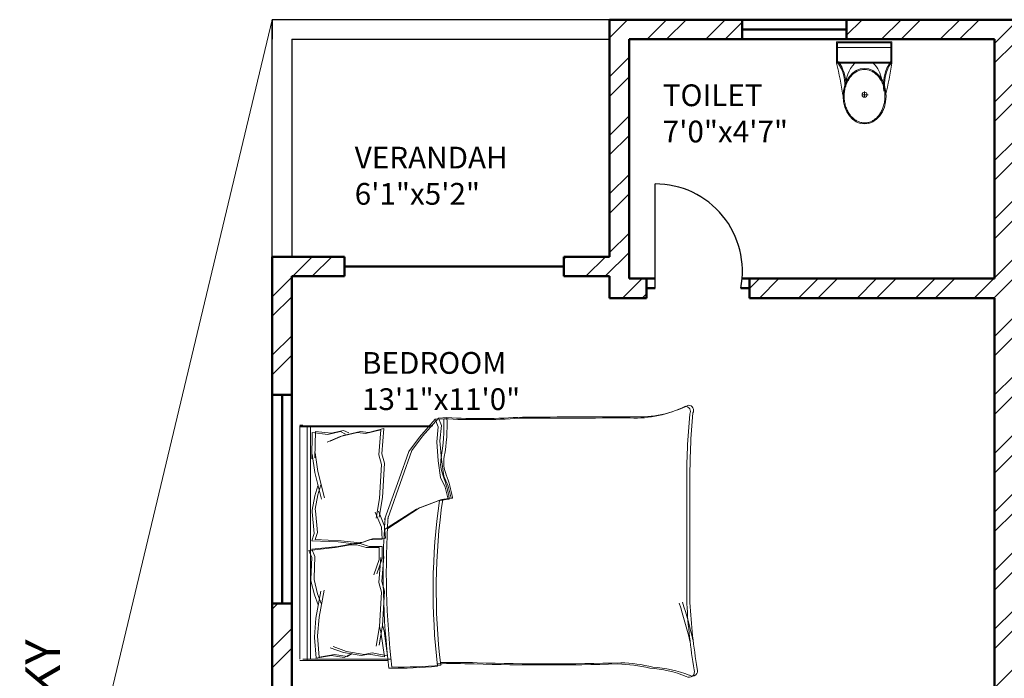
# Model space of a CAD drawing. Units: inches. Extents: x 1901 to 2863, y 888 to 2433.
# Tile 78 of 91: x 2381 to 2608, y 2123 to 2274. Entities that reach past the tile are written whole.
import ezdxf

# ---------------------------------------------------------------- set-up
doc = ezdxf.new("R2010")
doc.units = ezdxf.units.IN
for name, color, linetype, lineweight in [('A-ANNO-SYMB', 8, 'Continuous', 13), ('A-AREA-IDEN', 7, 'Continuous', 18), ('A-DOOR', 4, 'Continuous', 25), ('A-FLOR-FIXT', 9, 'Continuous', 18), ('A-FLOR-HRAL', 41, 'Continuous', 25), ('A-FURN', 8, 'Continuous', 18), ('A-WALL', 7, 'Continuous', 50), ('A-WALL-PATT', 8, 'Continuous', 13)]:
    doc.layers.add(name, color=color, linetype=linetype, lineweight=lineweight)
doc.styles.get("Standard").update_dxf_attribs({"font": 'arial.ttf'})

# ---------------------------------------------------------------- blocks, each defined once
blk = doc.blocks.new('A$C31115884')
for p, q in [((283.1, 497.7), (223.4, 497.7)), ((257.5, 466.4), (257.5, 523.2)), ((0, 200), (0, 0)), ((520, 200), (0, 200)), ((10, 190), (10, 10)), ((510, 190), (10, 190)), ((510, 10), (510, 190)), ((520, 0), (520, 200)), ((510, 54.5), (0, 54.5)), ((10, 10), (510, 10)), ((0, 0), (520, 0))]:
    blk.add_line(p, q)
blk.add_circle((255.6, 496.4), 23.6)
for centre, radius, start, end in [((2777.7, -204.6), 2807, 165.4549, 171.71327), ((-294.5, 403.3), 364.7, 324.20913, 9.34987), ((-294.5, 403.3), 374.7, 324.20913, 9.34987), ((805.8, 403.3), 364.7, 170.65013, 215.79087), ((3237, 905), 2807, 188.28673, 194.5451), ((139.5, 406.2), 293.5, 315.84364, 2.65635), ((805.8, 403.3), 374.7, 179.20365, 215.79087), ((383.6, 406.2), 293.5, 190.27735, 224.15636)]:
    blk.add_arc(centre, radius, start, end)
blk.add_ellipse((256.2, 509.9), major_axis=(0, -260.7), ratio=0.772727)
blk.add_open_spline([(256.2, 259.2), (263.1, 259.2), (270, 259.7), (287.8, 262.3), (298.7, 265.1), (319.9, 273.1), (330.2, 278.4), (350.1, 291.1), (359.7, 298.7), (377.7, 315.9), (386.2, 325.5), (401.7, 346.6), (408.8, 358.1), (421.3, 382.5), (426.8, 395.5), (435.9, 422.4), (439.5, 436.4), (444.8, 465.1), (446.5, 479.7), (447.9, 509.2), (447.6, 524), (445, 553.3), (442.7, 567.8), (436.3, 596), (432.1, 609.7), (421.9, 636), (416, 648.6), (402.5, 672.1), (395, 683), (378.6, 703), (369.8, 712.1), (351.1, 728), (341.3, 734.8), (320.9, 746.2), (310.4, 750.7), (288.9, 757.3), (278, 759.4), (256, 761), (245, 760.6), (223.1, 757.2), (212.3, 754.3), (191.1, 746.1), (180.8, 740.7), (160.9, 727.8), (151.4, 720.1), (133.5, 702.7), (125.1, 693), (109.6, 671.7), (102.6, 660.2), (90.2, 635.7), (84.9, 622.7), (76, 595.6), (72.4, 581.6), (67.2, 552.9), (65.6, 538.2), (64.4, 508.8), (64.8, 494), (67.5, 464.7), (69.9, 450.2), (76.6, 422), (80.8, 408.3), (91.1, 382.2), (97.2, 369.7), (110.8, 346.3), (118.4, 335.4), (134.8, 315.6), (143.7, 306.7), (162.4, 290.9), (172.3, 284.2), (192.8, 273), (203.3, 268.6), (224.8, 262.2), (235.8, 260.2), (249.9, 259.3), (253, 259.2), (256.2, 259.2)], degree=3, knots=[0, 0, 0, 0, 0.110105, 0.110105, 0.285049, 0.285049, 0.459994, 0.459994, 0.634938, 0.634938, 0.809882, 0.809882, 0.984827, 0.984827, 1.159771, 1.159771, 1.334715, 1.334715, 1.50966, 1.50966, 1.684604, 1.684604, 1.859549, 1.859549, 2.034493, 2.034493, 2.209437, 2.209437, 2.384382, 2.384382, 2.559326, 2.559326, 2.73427, 2.73427, 2.909215, 2.909215, 3.084159, 3.084159, 3.259103, 3.259103, 3.434048, 3.434048, 3.608992, 3.608992, 3.783936, 3.783936, 3.958881, 3.958881, 4.133825, 4.133825, 4.30877, 4.30877, 4.483714, 4.483714, 4.658658, 4.658658, 4.833603, 4.833603, 5.008547, 5.008547, 5.183491, 5.183491, 5.358436, 5.358436, 5.53338, 5.53338, 5.708324, 5.708324, 5.883269, 5.883269, 6.058213, 6.058213, 6.233158, 6.233158, 6.283185, 6.283185, 6.283185, 6.283185])
blk = doc.blocks.new('BED-DOUBLE')
for p, q in [((31.18, 59.32), (27.53, 55.16)), ((31.18, 59.32), (27.53, 55.16)), ((31.9, 59.58), (28.25, 55.42)), ((31.9, 59.58), (28.25, 55.42)), ((33.14, 59.41), (31.18, 59.32, 4.35)), ((33.14, 59.41), (31.18, 59.32, 4.35)), ((31.87, 57.59), (31.18, 59.32)), ((31.87, 57.59), (31.18, 59.32)), ((33.85, 59.67), (31.9, 59.58, 4.35)), ((33.85, 59.67), (31.9, 59.58, 4.35)), ((32.59, 57.85), (31.9, 59.58)), ((32.59, 57.85), (31.9, 59.58)), ((0.03, 57.78), (0.03, 4.12)), ((0.74, 57.78), (30.62, 57.78)), ((0.74, 57.78), (30.62, 57.78)), ((7.22, 56.06), (10.11, 56.73)), ((7.22, 56.06), (10.11, 56.73)), ((10.11, 56.73), (11.28, 56.15)), ((10.11, 56.73), (11.28, 56.15)), ((18.63, 56.89), (15.11, 56.01)), ((18.63, 56.88), (15.11, 56.01)), ((19.35, 57.14), (15.83, 56.27)), ((19.35, 57.14), (15.83, 56.27)), ((18.18, 51.12), (18.63, 56.89)), ((18.18, 51.12), (18.63, 56.88)), ((18.9, 51.38), (19.35, 57.14)), ((18.9, 51.38), (19.35, 57.14)), ((31.53, 54.12), (31.87, 57.59)), ((31.53, 54.12), (31.87, 57.59)), ((32.24, 54.37), (32.59, 57.85)), ((32.24, 54.37), (32.59, 57.85)), ((2.9, 56.23), (2.79, 50.16)), ((2.9, 56.23), (2.79, 50.16)), ((2.9, 56.23), (6.5, 55.8)), ((2.9, 56.23), (6.5, 55.8)), ((3.61, 56.48), (3.51, 50.42)), ((3.61, 56.48), (3.51, 50.42)), ((3.61, 56.48), (7.22, 56.06)), ((3.61, 56.48), (7.22, 56.06)), ((9.3, 55.33), (6.29, 54)), ((9.3, 55.33), (6.29, 54)), ((6.5, 55.8), (9.39, 56.47)), ((6.5, 55.8), (9.39, 56.47)), ((10.01, 55.58), (7.01, 54.26)), ((10.01, 55.58), (7.01, 54.26)), ((13.31, 56.23), (9.3, 55.33)), ((13.31, 56.23), (9.3, 55.33)), ((9.39, 56.47), (10.56, 55.89)), ((9.39, 56.47), (10.56, 55.89)), ((14.02, 56.48), (10.01, 55.58)), ((14.02, 56.48), (10.01, 55.58)), ((15.11, 56.01), (13.31, 56.23)), ((15.11, 56.01), (13.31, 56.23)), ((15.83, 56.27), (14.02, 56.48)), ((15.83, 56.27), (14.02, 56.48)), ((27.53, 55.16), (25.1, 51.86)), ((27.53, 55.16), (25.1, 51.86)), ((28.25, 55.42), (25.81, 52.11)), ((28.25, 55.42), (25.81, 52.11)), ((32.59, 50.03), (32.24, 54.37)), ((32.59, 50.03), (32.24, 54.37)), ((25.81, 52.11), (23.55, 45.85)), ((25.81, 52.11), (23.55, 45.85)), ((31.87, 49.77), (31.53, 54.12)), ((31.87, 49.77), (31.53, 54.12)), ((2.79, 50.16), (2.88, 51.29)), ((2.79, 50.16), (2.88, 51.29)), ((2.88, 51.29), (3.47, 47.02)), ((2.88, 51.29), (3.47, 47.02)), ((3.51, 50.42), (3.6, 51.54)), ((3.51, 50.42), (3.6, 51.54)), ((3.6, 51.54), (4.19, 47.28)), ((3.6, 51.54), (4.19, 47.28)), ((18.81, 48.92), (18.18, 51.12)), ((18.81, 48.92), (18.18, 51.12)), ((19.52, 49.18), (18.9, 51.38)), ((19.52, 49.18), (18.9, 51.38)), ((25.1, 51.86), (22.84, 45.6)), ((25.1, 51.86), (22.84, 45.6)), ((33.11, 46.2), (32.59, 50.03)), ((33.11, 46.2), (32.59, 50.03)), ((18.32, 41.05), (18.81, 48.92)), ((18.32, 41.05), (18.81, 48.92)), ((19.04, 41.31), (19.52, 49.18)), ((19.04, 41.31), (19.52, 49.18)), ((32.39, 45.94), (31.87, 49.77)), ((32.39, 45.94), (31.87, 49.77)), ((3.47, 47.02), (4.99, 40.94)), ((3.47, 47.02), (4.99, 40.94)), ((4.19, 47.28), (5.71, 41.19)), ((4.19, 47.28), (5.71, 41.19)), ((22.84, 45.6), (19.54, 36.24)), ((22.84, 45.6), (19.54, 36.24)), ((23.55, 45.85), (20.26, 36.49)), ((23.55, 45.85), (20.26, 36.49)), ((33.44, 43.68), (32.39, 45.94)), ((33.44, 43.68), (32.39, 45.94)), ((34.15, 43.94), (33.11, 46.2)), ((34.15, 43.94), (33.11, 46.2)), ((4.15, 43.98), (3.48, 41.66)), ((4.15, 43.98), (3.48, 41.66)), ((4.87, 44.23), (4.2, 41.91)), ((4.87, 44.23), (4.2, 41.91)), ((34.13, 40.9), (33.44, 43.68)), ((34.13, 40.9), (33.44, 43.68)), ((34.85, 41.16), (34.15, 43.94)), ((34.85, 41.16), (34.15, 43.94)), ((89, 16.88), (89, 44.51)), ((89, 16.88), (89, 44.51)), ((89.72, 17.13), (89.72, 44.77)), ((89.72, 17.13), (89.72, 44.77)), ((3.48, 41.66), (2.87, 38.37)), ((3.48, 41.66), (2.87, 38.37)), ((4.2, 41.91), (3.59, 38.62)), ((4.2, 41.91), (3.59, 38.62)), ((17.57, 36.53), (18.32, 41.05)), ((17.57, 36.52), (18.32, 41.05)), ((18.29, 36.78), (19.04, 41.31)), ((18.29, 36.78), (19.04, 41.31)), ((27.55, 38.9), (32.59, 40.81)), ((27.55, 38.9), (32.59, 40.81)), ((31.87, 40.55), (34.13, 40.9)), ((31.87, 40.55), (34.13, 40.9)), ((32.59, 40.81), (34.85, 41.16)), ((32.59, 40.81), (34.85, 41.16)), ((3.59, 38.62), (3.62, 38.26)), ((3.59, 38.62), (3.62, 38.26)), ((19.54, 33.94), (26.83, 38.64)), ((19.54, 33.94), (26.83, 38.64)), ((20.26, 34.19), (27.55, 38.9)), ((20.26, 34.19), (27.55, 38.9)), ((26.83, 38.64), (31.87, 40.55)), ((26.83, 38.64), (31.87, 40.55)), ((2.87, 38.37), (2.9, 38.01)), ((2.87, 38.37), (2.9, 38.01)), ((2.9, 38.01), (3.37, 33.03)), ((2.9, 38.01), (3.37, 33.04)), ((3.62, 38.26), (4.09, 33.29)), ((3.62, 38.26), (4.09, 33.29)), ((18.82, 34.49), (17.38, 37.94)), ((18.82, 34.49), (17.38, 37.94)), ((19.54, 34.74), (18.1, 38.19)), ((19.54, 34.74), (18.1, 38.19)), ((18.99, 31.73), (18.82, 34.49)), ((18.99, 31.73), (18.82, 34.49)), ((19.71, 31.99), (19.54, 34.74)), ((19.71, 31.99), (19.54, 34.74)), ((3.37, 33.04), (2.82, 31.37)), ((3.37, 33.03), (2.82, 31.37)), ((4.09, 33.29), (3.54, 31.63)), ((4.09, 33.29), (3.54, 31.63)), ((14.64, 31.02), (16.71, 31.8)), ((14.64, 31.02), (16.71, 31.8)), ((15.99, 31.55), (18.99, 31.73)), ((15.99, 31.55), (18.99, 31.73)), ((16.71, 31.8), (19.71, 31.99)), ((16.71, 31.8), (19.71, 31.99)), ((2.13, 29.14), (8.13, 29.78)), ((2.13, 29.14), (8.13, 29.78)), ((2.82, 31.37), (8.86, 31.1)), ((2.82, 31.37), (8.86, 31.1)), ((2.84, 29.39), (8.85, 30.04)), ((2.84, 29.39), (8.85, 30.04)), ((3.54, 31.63), (9.58, 31.36)), ((3.54, 31.63), (9.58, 31.36)), ((8.13, 29.78), (11.7, 30.43)), ((8.13, 29.78), (11.7, 30.43)), ((8.85, 30.04), (12.42, 30.69)), ((8.85, 30.04), (12.42, 30.69)), ((8.86, 31.1), (12.46, 30.68)), ((8.86, 31.1), (12.46, 30.68)), ((9.58, 31.36), (13.18, 30.93)), ((9.58, 31.36), (13.18, 30.93)), ((11.7, 30.43), (13.16, 30.43)), ((11.7, 30.43), (13.16, 30.43)), ((12.42, 30.69), (13.88, 30.69)), ((12.42, 30.69), (13.88, 30.69)), ((12.46, 30.68), (13.92, 30.77)), ((12.46, 30.68), (13.92, 30.77)), ((13.16, 30.43), (15.28, 29.78)), ((13.16, 30.43), (15.28, 29.78)), ((13.18, 30.93), (14.64, 31.02)), ((13.18, 30.93), (14.64, 31.02)), ((13.88, 30.69), (15.99, 30.04)), ((13.88, 30.69), (15.99, 30.04)), ((13.92, 30.77), (15.99, 31.55)), ((13.92, 30.77), (15.99, 31.55)), ((15.28, 29.78), (18.29, 29.78)), ((15.28, 29.78), (18.29, 29.78)), ((15.99, 30.04), (19, 30.04)), ((15.99, 30.04), (19, 30.04)), ((18.29, 29.78), (18.29, 27.03)), ((18.29, 29.78), (18.29, 27.03)), ((19, 30.04), (19, 27.28)), ((19, 30.04), (19, 27.28)), ((2.78, 27.51), (2.13, 29.14)), ((2.78, 27.51), (2.13, 29.14)), ((2.61, 22.52), (2.78, 27.51)), ((2.61, 22.52), (2.78, 27.51)), ((3.49, 27.77), (2.84, 29.39)), ((3.49, 27.77), (2.84, 29.39)), ((3.33, 22.78), (3.49, 27.77)), ((3.33, 22.78), (3.49, 27.77)), ((19, 27.28), (17.78, 23.75)), ((19, 27.28), (17.78, 23.75)), ((18.18, 21.73), (18.63, 27.49)), ((18.18, 21.73), (18.63, 27.49)), ((18.9, 21.98), (19.35, 27.75)), ((18.9, 21.98), (19.35, 27.74)), ((18.29, 27.03), (17.06, 23.49)), ((18.29, 27.03), (17.06, 23.5)), ((3.33, 22.42), (3.33, 22.78)), ((3.33, 22.42), (3.33, 22.78)), ((2.61, 22.16), (2.61, 22.52)), ((2.61, 22.16), (2.61, 22.52)), ((3.42, 18.91), (2.61, 22.16)), ((3.42, 18.91), (2.61, 22.16)), ((4.14, 19.17), (3.33, 22.42)), ((4.14, 19.17), (3.33, 22.42)), ((18.81, 19.53), (18.18, 21.73)), ((18.81, 19.53), (18.18, 21.73)), ((19.52, 19.78), (18.9, 21.98)), ((19.52, 19.78), (18.9, 21.98)), ((4.24, 16.64), (3.42, 18.91)), ((4.24, 16.64), (3.42, 18.91)), ((3.75, 13.56), (4.89, 19.73)), ((3.75, 13.56), (4.89, 19.73)), ((4.95, 16.9), (4.14, 19.17)), ((4.95, 16.9), (4.14, 19.17)), ((4.47, 13.81), (5.6, 19.98)), ((4.47, 13.81), (5.6, 19.98)), ((18.32, 11.66), (18.81, 19.53)), ((18.32, 11.66), (18.81, 19.53)), ((19.04, 11.91), (19.52, 19.78)), ((19.04, 11.91), (19.52, 19.78)), ((4.14, 9.52), (4.47, 13.81)), ((4.14, 9.52), (4.47, 13.81)), ((3.42, 9.27), (3.75, 13.56)), ((3.42, 9.27), (3.75, 13.56)), ((17.57, 7.13), (18.32, 11.66)), ((17.57, 7.13), (18.32, 11.66)), ((18.29, 7.38), (19.04, 11.91)), ((18.29, 7.39), (19.04, 11.91)), ((18.32, 11.66), (18.68, 10.38)), ((18.32, 11.66), (18.68, 10.38)), ((19.04, 11.91), (19.4, 10.64)), ((19.04, 11.91), (19.4, 10.64)), ((3.4, 9.15), (3.42, 9.27)), ((3.4, 9.15), (3.42, 9.27)), ((3.77, 4.34), (3.4, 9.15)), ((3.77, 4.34), (3.4, 9.15)), ((4.12, 9.4), (4.14, 9.52)), ((4.12, 9.4), (4.14, 9.52)), ((4.49, 4.6), (4.12, 9.4)), ((4.49, 4.6), (4.12, 9.4)), ((18.68, 10.38), (19.5, 4.66)), ((18.68, 10.38), (19.5, 4.66)), ((19.4, 10.64), (20.21, 4.92)), ((19.4, 10.64), (20.21, 4.92)), ((10.8, 5.89), (7.71, 7.03)), ((10.8, 5.89), (7.71, 7.03)), ((3.75, 4.34), (7.32, 4.99)), ((3.75, 4.34), (7.32, 4.99)), ((4.47, 4.59), (8.04, 5.24)), ((4.47, 4.59), (8.04, 5.24)), ((10.08, 5.63), (7, 6.77)), ((10.08, 5.63), (7, 6.77)), ((7.32, 4.99), (10.24, 4.5)), ((7.32, 4.99), (10.24, 4.5)), ((8.04, 5.24), (10.96, 4.75)), ((8.04, 5.24), (10.96, 4.76)), ((14.14, 4.99), (10.08, 5.63)), ((14.14, 4.99), (10.08, 5.63)), ((10.24, 4.5), (11.38, 5.15)), ((10.24, 4.5), (11.38, 5.15)), ((14.86, 5.24), (10.8, 5.89)), ((14.86, 5.24), (10.8, 5.89)), ((10.96, 4.76), (12.1, 5.4)), ((10.96, 4.75), (12.1, 5.4)), ((15.92, 5.31), (14.14, 4.99)), ((15.92, 5.31), (14.14, 4.99)), ((16.64, 5.57), (14.86, 5.24)), ((16.64, 5.57), (14.86, 5.24)), ((19.5, 4.66), (15.92, 5.31)), ((19.5, 4.66), (15.92, 5.31)), ((20.21, 4.92), (16.64, 5.57)), ((20.21, 4.92), (16.64, 5.57))]:
    blk.add_line(p, q)
for centre, radius, start, end in [((77.12, 85.47), 25.9, 267.4714, 296.4681), ((77.12, 85.47), 25.9, 267.4714, 296.4681), ((77.84, 85.73), 25.9, 267.4714, 296.4681), ((77.84, 85.73), 25.9, 267.4714, 296.4681), ((88.58, 61.05), 1.24, 332.6588, 86.02), ((88.58, 61.05), 1.24, 332.6588, 86.02), ((89.3, 61.31), 1.24, 332.6588, 86.02), ((89.3, 61.31), 1.24, 332.6588, 86.02), ((-7.45, 57.59), 40.62, 349.8763, 2.5657), ((-7.45, 57.59), 40.62, 349.8763, 2.5657), ((40.8, 204.6), 145.39, 266.9791, 273.8365), ((40.8, 204.6), 145.39, 266.9791, 273.8365), ((-6.73, 57.85), 40.62, 349.8763, 2.5657), ((-6.73, 57.85), 40.62, 349.8763, 2.5657), ((41.52, 204.86), 145.39, 266.9791, 273.8365), ((41.52, 204.86), 145.39, 266.9791, 273.8365), ((76.17, -5062.23), 5121.82, 90.00217, 90.28689), ((76.17, -5062.23), 5121.82, 90.00217, 90.28689), ((76.89, -5061.97), 5121.82, 90.00217, 90.28689), ((76.89, -5061.97), 5121.82, 90.00217, 90.28689), ((238.36, 46.17), 149.37, 174.4998, 180.6351), ((238.36, 46.17), 149.37, 174.4998, 180.6351), ((239.08, 46.42), 149.37, 174.4998, 180.6351), ((239.08, 46.42), 149.37, 174.4998, 180.6351), ((39.4, 49.08), 6.99, 168.6608, 203.7384), ((39.4, 49.08), 6.99, 168.6608, 203.7384), ((40.11, 49.33), 6.99, 168.6608, 203.7384), ((40.11, 49.33), 6.99, 168.6608, 203.7384), ((1.69, 34.94), 33.29, 10.6617, 19.8806), ((1.69, 34.94), 33.29, 10.6617, 19.8806), ((2.41, 35.2), 33.29, 10.6617, 19.8806), ((2.41, 35.2), 33.29, 10.6617, 19.8806), ((176.25, 20.16), 144.86, 171.7845, 186.9006), ((176.25, 20.15), 144.86, 171.7845, 186.9006), ((34.2, 41.1), 0.207, 250.2464, 1.1377), ((34.2, 41.1), 0.207, 250.2464, 1.1377), ((34.92, 41.35), 0.207, 250.2464, 1.1377), ((34.92, 41.35), 0.207, 250.2464, 1.1377), ((175.53, 19.9), 144.86, 171.7845, 186.9006), ((175.53, 19.9), 144.86, 171.7845, 186.9006), ((204.43, 23.94), 185.22, 176.0865, 186.7821), ((204.43, 23.94), 185.22, 176.0865, 186.7821), ((205.14, 24.2), 185.22, 176.0865, 186.7821), ((205.14, 24.2), 185.22, 176.0865, 186.7821), ((225.52, 24.02), 136.7, 182.9958, 189.4091), ((225.52, 24.02), 136.7, 182.9958, 189.4091), ((226.23, 24.28), 136.7, 182.9958, 189.4091), ((226.23, 24.28), 136.7, 182.9958, 189.4091), ((22.59, 95.58), 93.53, 268.7218, 275.604), ((22.59, 95.58), 93.53, 268.7218, 275.604), ((23.31, 95.84), 93.53, 268.7218, 275.604), ((23.31, 95.84), 93.53, 268.7218, 275.604), ((35.03, -187.88), 190.99, 88.4762, 91.0082), ((35.03, -187.88), 190.99, 88.4762, 91.0082), ((35.74, -187.62), 190.99, 88.4762, 91.0082), ((35.74, -187.62), 190.99, 88.4762, 91.0082), ((56.85, 544.3), 541.51, 268.2277, 271.7185), ((56.85, 544.3), 541.51, 268.2277, 271.7185), ((57.57, 544.55), 541.51, 268.2277, 271.7185), ((57.57, 544.55), 541.51, 268.2277, 271.7185), ((72.46, -30.24), 33.27, 76.0648, 88.9113), ((72.46, -30.24), 33.27, 76.0648, 88.9113), ((73.18, -29.98), 33.27, 76.0648, 88.9113), ((73.18, -29.98), 33.27, 76.0648, 88.9113), ((79.65, -24.1), 26.45, 67.9751, 86.652), ((79.65, -24.1), 26.45, 67.9751, 86.652), ((78.93, -24.35), 26.45, 67.9751, 86.652), ((78.93, -24.35), 26.45, 67.9751, 86.652), ((89.53, 1.18), 1.22, 236.1736, 23.4781), ((89.53, 1.18), 1.22, 236.1736, 23.4781), ((90.25, 1.44), 1.22, 236.1736, 23.4781), ((90.25, 1.44), 1.22, 236.1736, 23.4781)]:
    blk.add_arc(centre, radius, start, end)
blk = doc.blocks.new('DOOR-20B')
blk.add_line((0, -0.02), (0, 23.98))
blk.add_arc((0, 3.9), 20.08, 348.7487, 90)

msp = doc.modelspace()

# ---------------------------------------------------------------- hatches: boundary and pattern name
at = {"layer": 'A-WALL-PATT'}
h = msp.add_hatch(dxfattribs=at)
h.set_pattern_fill('ANSI32', color=256)
h.paths.add_polyline_path([(2192.5, 2274.13), (2141.26, 2274.13), (2141.26, 2269.63), (2192.5, 2269.63)])
h.paths.add_polyline_path([(2259.93, 2274.13), (2216.5, 2274.13), (2216.5, 2269.63), (2255.43, 2269.63), (2255.43, 2214.63), (2250.81, 2214.63), (2250.81, 2210.13), (2259.93, 2210.13), (2259.93, 2215.13), (2271.76, 2215.13), (2271.76, 2217.38), (2271.76, 2219.63), (2259.93, 2219.63)])
h.paths.add_polyline_path([(2171.43, 2269.63), (2166.93, 2269.63), (2166.93, 2219.63), (2121.24, 2219.63), (2121.24, 2215.13), (2166.93, 2215.13), (2166.93, 2083.13), (2161.81, 2083.13), (2161.81, 2078.63), (2171.43, 2078.63), (2177, 2078.63), (2177, 2080.88), (2177, 2083.13), (2171.43, 2083.13), (2171.43, 2210.13), (2230.91, 2210.13), (2230.91, 2212.38), (2230.91, 2214.63), (2171.43, 2214.63)])
h.paths.add_polyline_path([(2117.26, 2274.13), (2089.43, 2274.13), (2089.43, 2219.63), (2081.14, 2219.63), (2081.14, 2215.13), (2089.43, 2215.13), (2098, 2215.13), (2098, 2217.38), (2098, 2219.63), (2093.93, 2219.63), (2093.93, 2269.63), (2117.26, 2269.63), (2117.26, 2271.88)])
h.paths.add_polyline_path([(2343.43, 2219.63), (2329.29, 2219.63), (2329.29, 2215.13), (2338.93, 2215.13), (2338.93, 2184.74), (2343.43, 2184.74)])
h.paths.add_polyline_path([(2338.93, 2083.13), (2329.29, 2083.13), (2208.97, 2083.13), (2208.97, 2078.63), (2338.93, 2078.63)])
h.paths.add_polyline_path([(2343.43, 2136.74), (2338.93, 2136.74), (2338.93, 1872.63), (2343.43, 1872.63)])
h.paths.add_polyline_path([(2343.43, 1863.63), (2397.68, 1863.63), (2397.68, 1821.63), (2384.14, 1821.63), (2384.14, 1812.63), (2418.33, 1812.63), (2418.33, 1817.13), (2418.33, 1821.63), (2406.68, 1821.63), (2406.68, 1863.63), (2459.5, 1863.63), (2459.5, 1821.63), (2447.14, 1821.63), (2447.14, 1812.63), (2459.5, 1812.63), (2468.5, 1812.63), (2468.5, 1872.63), (2394.43, 1872.63), (2334.43, 1872.63), (2334.43, 1812.63), (2343.43, 1812.63), (2353.25, 1812.63), (2353.25, 1821.63), (2343.43, 1821.63)])
h.paths.add_polyline_path([(2510.01, 1872.63), (2468.5, 1872.63), (2468.5, 1868.13), (2510.01, 1868.13)])
h.paths.add_polyline_path([(2514.01, 1817.13), (2468.5, 1817.13), (2468.5, 1812.63), (2482.11, 1812.63), (2482.11, 1800.61), (2486.61, 1800.61), (2486.61, 1812.63), (2514.01, 1812.63)])
h.paths.add_polyline_path([(2299.25, 1814.88), (2299.25, 1817.13), (2295.93, 1817.13), (2295.93, 1854.17), (2293.68, 1854.17), (2291.43, 1854.17), (2291.43, 1817.13), (2266.11, 1817.13), (2266.11, 1812.63), (2299.25, 1812.63)])
h.paths.add_polyline_path([(2218.11, 1817.13), (2206.46, 1817.13), (2171.43, 1817.13), (2171.43, 1949.13), (2190.1, 1949.13), (2190.1, 1953.63), (2163.47, 1953.63), (2163.47, 1949.13), (2166.93, 1949.13), (2166.93, 1817.13), (2114.3, 1817.13), (2114.3, 1812.63), (2218.11, 1812.63)])
h.paths.add_polyline_path([(2029.43, 1970.92), (2024.93, 1970.92), (2024.93, 1912.72), (2029.43, 1912.72)])
h.paths.add_polyline_path([(2132.3, 1953.63), (2113.93, 1953.63), (2113.93, 1975.89), (2111.68, 1975.89), (2109.43, 1975.89), (2109.43, 1953.63), (2029.43, 1953.63), (2029.43, 1949.13), (2132.3, 1949.13)])
h.paths.add_polyline_path([(2029.43, 1853.61), (2029.31, 1853.61), (2029.31, 1853.61), (2029.43, 1853.61), (2029.43, 1864.72), (2024.93, 1864.72), (2024.93, 1812.63), (2066.3, 1812.63), (2066.3, 1814.88), (2066.3, 1817.13), (2029.43, 1817.13)])
h.paths.add_polyline_path([(2122.93, 2010.09), (2120.68, 2010.09), (2118.43, 2010.09), (2118.43, 2006.13), (2029.43, 2006.13), (2029.43, 2001.63), (2109.43, 2001.63), (2109.43, 1998.04), (2113.93, 1998.04), (2113.93, 2001.63), (2122.93, 2001.63)])
h.paths.add_polyline_path([(2029.43, 2031.38), (2024.93, 2031.38), (2024.93, 1994.92), (2027.18, 1994.92), (2029.43, 1994.92)])
h.paths.add_polyline_path([(2029.43, 2136.74), (2024.93, 2136.74), (2024.93, 2067.38), (2027.18, 2067.38), (2029.43, 2067.38)])
h.paths.add_polyline_path([(2125.62, 2083.13), (2029.43, 2083.13), (2029.43, 2078.63), (2118.43, 2078.63), (2118.43, 2030.71), (2122.93, 2030.71), (2122.93, 2078.63), (2125.62, 2078.63)])
h.paths.add_polyline_path([(2029.43, 2215.13), (2040.47, 2215.13), (2040.47, 2217.38), (2040.47, 2219.63), (2024.93, 2219.63), (2024.93, 2184.74), (2029.43, 2184.74), (2029.43, 2187.78)])
h.paths.add_polyline_path([(2686.43, 2274.13), (2659.28, 2274.13), (2659.28, 2269.63), (2681.93, 2269.63), (2681.93, 2219.63), (2676.82, 2219.63), (2676.82, 2215.13), (2681.93, 2215.13), (2697.01, 2215.13), (2697.01, 2217.38), (2697.01, 2219.63), (2686.43, 2219.63)])
h.paths.add_polyline_path([(2609.93, 2269.63), (2635.28, 2269.63), (2635.28, 2274.13), (2571.43, 2274.13), (2571.43, 2269.63), (2605.43, 2269.63), (2605.43, 2214.63), (2549.1, 2214.63), (2549.1, 2210.13), (2605.43, 2210.13), (2605.43, 2083.13), (2601.01, 2083.13), (2601.01, 2080.88), (2601.01, 2078.63), (2609.93, 2078.63), (2616.16, 2078.63), (2616.16, 2080.88), (2616.16, 2083.13), (2609.93, 2083.13), (2609.93, 2215.13), (2651.46, 2215.13), (2651.46, 2217.38), (2651.46, 2219.63), (2609.93, 2219.63)])
h.paths.add_polyline_path([(2521.43, 2269.63), (2547.43, 2269.63), (2547.43, 2271.88), (2547.43, 2274.13), (2516.93, 2274.13), (2516.93, 2219.63), (2506.41, 2219.63), (2506.41, 2215.13), (2516.93, 2215.13), (2516.93, 2210.13), (2525.4, 2210.13), (2525.4, 2212.38), (2525.4, 2214.63), (2521.43, 2214.63)])
h.paths.add_polyline_path([(2456.01, 2219.63), (2439.43, 2219.63), (2439.43, 2187.89), (2443.93, 2187.89), (2443.93, 2215.13), (2456.01, 2215.13)])
h.paths.add_polyline_path([(2752.93, 2219.63), (2739.48, 2219.63), (2739.48, 2215.13), (2748.43, 2215.13), (2748.43, 2187.89), (2752.93, 2187.89)])
h.paths.add_polyline_path([(2752.93, 2139.89), (2748.43, 2139.89), (2748.43, 2083.13), (2648.42, 2083.13), (2648.42, 2078.63), (2654.93, 2078.63), (2654.93, 2039.44), (2659.43, 2039.44), (2659.43, 2078.63), (2748.43, 2078.63), (2748.43, 2063.43), (2752.93, 2063.43)])
h.paths.add_polyline_path([(2752.93, 2010.63), (2659.43, 2010.63), (2659.43, 2015.65), (2654.93, 2015.65), (2654.93, 2010.63), (2605.43, 2010.63), (2605.43, 1920.97), (2609.93, 1920.97), (2609.93, 2006.13), (2748.43, 2006.13), (2748.43, 1982.47), (2752.93, 1982.47)])
h.paths.add_polyline_path([(2752.93, 2027.43), (2748.43, 2027.43), (2748.43, 2010.63), (2752.93, 2010.63)])
h.paths.add_polyline_path([(2748.43, 1886.13), (2609.93, 1886.13), (2609.93, 1889.72), (2605.43, 1889.72), (2605.43, 1861.26), (2609.93, 1861.26), (2609.93, 1881.63), (2748.43, 1881.63)])
h.paths.add_polyline_path([(2456.86, 2228.83), (2498.4, 2228.83), (2498.4, 2247.49), (2456.86, 2247.49)], flags=9)
h.paths.add_polyline_path([(2038.6, 2237.42), (2080.17, 2237.42), (2080.17, 2256.08), (2038.6, 2256.08)], flags=9)
h.paths.add_polyline_path([(2292.01, 1062.39), (2539.93, 1062.39), (2539.93, 1099.49), (2292.01, 1099.49)], flags=9)
h.paths.add_polyline_path([(2424.91, 1832.25), (2448.51, 1832.25), (2448.51, 1846.68), (2424.91, 1846.68)], flags=25)
h.paths.add_polyline_path([(2359.08, 1832.25), (2382.68, 1832.25), (2382.68, 1846.68), (2359.08, 1846.68)], flags=25)
h.paths.add_polyline_path([(2352.9, 1684.8), (2367.54, 1684.8), (2367.54, 1697.17), (2352.9, 1697.17)], flags=9)
h.paths.add_polyline_path([(2079.29, 1755.83), (2169.02, 1755.83), (2169.02, 1774.37), (2079.29, 1774.37)], flags=9)
h.paths.add_polyline_path([(2404.09, 1373.86), (2404.09, 1463.59), (2385.54, 1463.59), (2385.54, 1373.86)], flags=9)
h.paths.add_polyline_path([(2268.09, 2236.37), (2309.64, 2236.37), (2309.64, 2255.03), (2268.09, 2255.03)], flags=9)
h.paths.add_polyline_path([(2575.96, 1700.95), (2665.7, 1700.95), (2665.7, 1719.5), (2575.96, 1719.5)], flags=9)
h.paths.add_polyline_path([(2302.96, 1878.47), (2329.52, 1878.47), (2329.52, 1888.78), (2302.96, 1888.78)], flags=9)
h.paths.add_polyline_path([(2097.42, 2240.58), (2126.57, 2240.58), (2126.57, 2259.23), (2097.42, 2259.23)], flags=9)
h.paths.add_polyline_path([(2208.72, 2246.12), (2237.88, 2246.12), (2237.88, 2264.78), (2208.72, 2264.78)], flags=9)
h.paths.add_polyline_path([(2038.15, 1925.96), (2076.99, 1925.96), (2076.99, 1944.62), (2038.15, 1944.62)], flags=9)
h.paths.add_polyline_path([(2239.14, 1926.67), (2288.46, 1926.67), (2288.46, 1945.33), (2239.14, 1945.33)], flags=9)
h.paths.add_polyline_path([(2175.43, 2007.33), (2212.36, 2007.33), (2212.36, 2025.99), (2175.43, 2025.99)], flags=9)
h.paths.add_polyline_path([(2225.03, 2091.79), (2263.87, 2091.79), (2263.87, 2110.45), (2225.03, 2110.45)], flags=9)
h.paths.add_polyline_path([(2035.4, 2098.48), (2074.24, 2098.48), (2074.24, 2117.14), (2035.4, 2117.14)], flags=9)
h.paths.add_polyline_path([(2050.1, 2029.21), (2083.26, 2029.21), (2083.26, 2047.87), (2050.1, 2047.87)], flags=9)
h.paths.add_polyline_path([(2069.68, 1956.72), (2098.83, 1956.72), (2098.83, 1975.38), (2069.68, 1975.38)], flags=25)
h.paths.add_polyline_path([(2328.62, 1753.34), (2361.66, 1753.34), (2361.66, 1771.99), (2328.62, 1771.99)], flags=9)
h.paths.add_polyline_path([(2395.16, 2060.89), (2395.16, 2140.65), (2378.68, 2140.65), (2378.68, 2060.89)], flags=9)
h.paths.add_polyline_path([(2463.73, 2059.02), (2492.89, 2059.02), (2492.89, 2077.68), (2463.73, 2077.68)], flags=9)
h.paths.add_polyline_path([(2458.03, 2181.54), (2496.87, 2181.54), (2496.87, 2200.19), (2458.03, 2200.19)], flags=9)
h.paths.add_polyline_path([(2527.58, 2243.07), (2556.73, 2243.07), (2556.73, 2261.73), (2527.58, 2261.73)], flags=9)
h.paths.add_polyline_path([(2694.46, 2232.77), (2736.03, 2232.77), (2736.03, 2251.42), (2694.46, 2251.42)], flags=9)
h.paths.add_polyline_path([(2637.82, 2249.22), (2666.98, 2249.22), (2666.98, 2267.88), (2637.82, 2267.88)], flags=9)
h.paths.add_polyline_path([(2623.69, 2183.54), (2662.53, 2183.54), (2662.53, 2202.2), (2623.69, 2202.2)], flags=9)
h.paths.add_polyline_path([(2691.97, 2021.5), (2725.12, 2021.5), (2725.12, 2040.16), (2691.97, 2040.16)], flags=9)
h.paths.add_polyline_path([(2621.04, 1975.91), (2662.34, 1975.91), (2662.34, 1994.57), (2621.04, 1994.57)], flags=25)
h.paths.add_polyline_path([(2479.03, 1927.62), (2519.84, 1927.62), (2519.84, 1946.28), (2479.03, 1946.28)], flags=9)
h.paths.add_polyline_path([(2670.94, 1849.08), (2716.01, 1849.08), (2716.01, 1867.73), (2670.94, 1867.73)], flags=9)
h.paths.add_polyline_path([(2523.61, 1782.96), (2550.17, 1782.96), (2550.17, 1793.26), (2523.61, 1793.26)], flags=9)
h.paths.add_polyline_path([(2450.84, 1207.33), (2492.39, 1207.33), (2492.39, 1225.99), (2450.84, 1225.99)], flags=9)
h.paths.add_polyline_path([(2527.75, 1203.84), (2556.91, 1203.84), (2556.91, 1222.5), (2527.75, 1222.5)], flags=9)
h.paths.add_polyline_path([(2639.11, 1207.2), (2668.27, 1207.2), (2668.27, 1225.86), (2639.11, 1225.86)], flags=9)
h.paths.add_polyline_path([(2692.59, 1218.97), (2734.17, 1218.97), (2734.17, 1237.62), (2692.59, 1237.62)], flags=9)
h.paths.add_polyline_path([(2669.27, 1366.33), (2708.11, 1366.33), (2708.11, 1384.99), (2669.27, 1384.99)], flags=9)
h.paths.add_polyline_path([(2463.31, 1358.03), (2502.15, 1358.03), (2502.15, 1376.69), (2463.31, 1376.69)], flags=9)
h.paths.add_polyline_path([(2494.72, 1449.96), (2531.65, 1449.96), (2531.65, 1468.62), (2494.72, 1468.62)], flags=9)
h.paths.add_polyline_path([(2675.57, 1422.16), (2708.72, 1422.16), (2708.72, 1440.81), (2675.57, 1440.81)], flags=9)
h.paths.add_polyline_path([(2685.63, 1493.89), (2714.79, 1493.89), (2714.79, 1512.55), (2685.63, 1512.55)], flags=9)
h.paths.add_polyline_path([(2686.8, 1529.91), (2725.65, 1529.91), (2725.65, 1548.57), (2686.8, 1548.57)], flags=9)
h.paths.add_polyline_path([(2503.65, 1537.99), (2552.97, 1537.99), (2552.97, 1556.65), (2503.65, 1556.65)], flags=9)
h.paths.add_polyline_path([(2291.71, 1643.5), (2318.28, 1643.5), (2318.28, 1653.81), (2291.71, 1653.81)], flags=9)
h.paths.add_polyline_path([(2450.63, 1610.52), (2477.19, 1610.52), (2477.19, 1620.82), (2450.63, 1620.82)], flags=9)
h.paths.add_polyline_path([(2359.99, 1551.81), (2422.25, 1551.81), (2422.25, 1562.12), (2359.99, 1562.12)], flags=9)
h.paths.add_polyline_path([(2280.11, 1249.01), (2321.65, 1249.01), (2321.65, 1267.66), (2280.11, 1267.66)], flags=9)
h.paths.add_polyline_path([(2164.06, 1274.23), (2193.22, 1274.23), (2193.22, 1292.89), (2164.06, 1292.89)], flags=9)
h.paths.add_polyline_path([(2118.21, 1277.69), (2151.25, 1277.69), (2151.25, 1296.35), (2118.21, 1296.35)], flags=9)
h.paths.add_polyline_path([(2031.95, 1268.53), (2073.52, 1268.53), (2073.52, 1287.19), (2031.95, 1287.19)], flags=9)
h.paths.add_polyline_path([(2050.2, 1409.08), (2089.04, 1409.08), (2089.04, 1427.74), (2050.2, 1427.74)], flags=9)
h.paths.add_polyline_path([(2243.74, 1421.03), (2282.58, 1421.03), (2282.58, 1439.69), (2243.74, 1439.69)], flags=9)
h.paths.add_polyline_path([(2190.75, 1509.77), (2231.56, 1509.77), (2231.56, 1528.43), (2190.75, 1528.43)], flags=9)
h.paths.add_polyline_path([(2058.39, 1475.42), (2091.55, 1475.42), (2091.55, 1494.07), (2058.39, 1494.07)], flags=9)
h.paths.add_polyline_path([(2062.45, 1553.09), (2091.6, 1553.09), (2091.6, 1571.75), (2062.45, 1571.75)], flags=9)
h.paths.add_polyline_path([(2219.52, 1590.37), (2266.15, 1590.37), (2266.15, 1609.02), (2219.52, 1609.02)], flags=9)
h.paths.add_polyline_path([(2041.07, 1584.19), (2079.91, 1584.19), (2079.91, 1602.85), (2041.07, 1602.85)], flags=9)
h = msp.add_hatch(dxfattribs=at)
h.set_pattern_fill('ANSI32', color=256)
h.paths.add_polyline_path([(2443.93, 2139.89), (2439.43, 2139.89), (2439.43, 2069.35), (2441.68, 2069.35), (2443.93, 2069.35), (2443.93, 2078.63), (2521.93, 2078.63), (2521.93, 2075.07), (2524.18, 2075.07), (2526.43, 2075.07), (2526.43, 2078.63), (2571.75, 2078.63), (2571.75, 2080.88), (2571.75, 2083.13), (2443.93, 2083.13)])
h.paths.add_polyline_path([(2526.43, 2054.63), (2524.18, 2054.63), (2521.93, 2054.63), (2521.93, 2030.63), (2443.93, 2030.63), (2443.93, 2045.35), (2439.43, 2045.35), (2439.43, 1983.87), (2443.93, 1983.87), (2443.93, 2026.13), (2521.93, 2026.13), (2526.43, 2026.13)])
h.paths.add_polyline_path([(2443.93, 1923.87), (2439.43, 1923.87), (2439.43, 1872.63), (2443.93, 1872.63)])
h.paths.add_polyline_path([(2636.23, 1766.13), (2609.93, 1766.13), (2609.93, 1779.79), (2605.43, 1779.79), (2605.43, 1766.13), (2486.61, 1766.13), (2486.61, 1770.67), (2482.11, 1770.67), (2482.11, 1766.13), (2482.11, 1761.63), (2636.23, 1761.63), (2636.23, 1763.88)])
h.paths.add_polyline_path([(2519.54, 1663.38), (2519.54, 1665.63), (2494.93, 1665.63), (2481.83, 1665.63), (2481.83, 1663.38), (2481.83, 1661.13), (2490.43, 1661.13), (2490.43, 1640.16), (2494.93, 1640.16), (2494.93, 1661.13), (2519.54, 1661.13)])
h.paths.add_polyline_path([(2443.93, 1712.13), (2443.93, 1716.63), (2414.46, 1716.63), (2414.46, 1712.13), (2439.43, 1712.13), (2439.43, 1545.51), (2443.93, 1545.51), (2443.93, 1661.13), (2448.47, 1661.13), (2448.47, 1665.63), (2443.93, 1665.63)])
h.paths.add_polyline_path([(2343.43, 1712.13), (2365.52, 1712.13), (2365.52, 1714.38), (2365.52, 1716.63), (2333.87, 1716.63), (2333.87, 1714.38), (2333.87, 1712.13), (2338.93, 1712.13), (2338.93, 1575.63), (2338.93, 1545.51), (2343.43, 1545.51), (2343.43, 1547.51), (2343.43, 1580.13)])
h.paths.add_polyline_path([(2752.93, 1665.63), (2579.54, 1665.63), (2579.54, 1661.13), (2615.93, 1661.13), (2615.93, 1529.13), (2598.93, 1529.13), (2598.93, 1524.63), (2623.13, 1524.63), (2623.13, 1526.88), (2623.13, 1529.13), (2620.43, 1529.13), (2620.43, 1661.13), (2748.43, 1661.13), (2748.43, 1633.5), (2752.93, 1633.5)])
h.paths.add_polyline_path([(2752.93, 1419.93), (2748.43, 1419.93), (2748.43, 1400.13), (2659.43, 1400.13), (2659.43, 1444.33), (2657.18, 1444.33), (2654.93, 1444.33), (2654.93, 1400.13), (2643.65, 1400.13), (2643.65, 1395.63), (2748.43, 1395.63), (2748.43, 1364.04), (2752.93, 1364.04)])
h.paths.add_polyline_path([(2752.93, 1492.88), (2748.43, 1492.88), (2748.43, 1476.63), (2667.43, 1476.63), (2667.43, 1479.71), (2665.18, 1479.71), (2662.93, 1479.71), (2662.93, 1476.63), (2654.93, 1476.63), (2654.93, 1469.54), (2659.43, 1469.54), (2659.43, 1472.13), (2748.43, 1472.13), (2748.43, 1455.93), (2752.93, 1455.93)])
h.paths.add_polyline_path([(2752.93, 1304.04), (2748.43, 1304.04), (2748.43, 1263.63), (2738.66, 1263.63), (2738.66, 1259.13), (2752.93, 1259.13)])
h.paths.add_polyline_path([(2685.93, 1259.13), (2695.49, 1259.13), (2695.49, 1261.38), (2695.49, 1263.63), (2677.84, 1263.63), (2677.84, 1261.38), (2677.84, 1259.13), (2681.43, 1259.13), (2681.43, 1203.63), (2653.28, 1203.63), (2653.28, 1199.13), (2685.93, 1199.13), (2685.93, 1203.63)])
h.paths.add_polyline_path([(2609.43, 1395.63), (2611.85, 1395.63), (2611.85, 1400.13), (2598.89, 1400.13), (2598.89, 1397.88), (2598.89, 1395.63), (2604.93, 1395.63), (2604.93, 1268.13), (2554.73, 1268.13), (2554.73, 1265.88), (2554.73, 1263.63), (2604.93, 1263.63), (2604.93, 1203.63), (2571.31, 1203.63), (2571.31, 1199.13), (2604.93, 1199.13), (2629.28, 1199.13), (2629.28, 1201.38), (2629.28, 1203.63), (2609.43, 1203.63), (2609.43, 1258.63), (2609.43, 1259.13), (2654.8, 1259.13), (2654.8, 1263.63), (2609.43, 1263.63)])
h.paths.add_polyline_path([(2443.93, 1304.04), (2439.43, 1304.04), (2439.43, 1259.13), (2443.93, 1259.13), (2456.16, 1259.13), (2456.16, 1261.38), (2456.16, 1263.63), (2443.93, 1263.63)])
h.paths.add_polyline_path([(2525.43, 1263.63), (2531.78, 1263.63), (2531.78, 1268.13), (2520.93, 1268.13), (2520.93, 1263.63), (2511.41, 1263.63), (2511.41, 1259.13), (2520.93, 1259.13), (2520.93, 1199.13), (2547.31, 1199.13), (2547.31, 1201.38), (2547.31, 1203.63), (2525.43, 1203.63)])
h.paths.add_polyline_path([(2443.93, 1434.84), (2439.43, 1434.84), (2439.43, 1364.04), (2441.68, 1364.04), (2443.93, 1364.04)])
h.paths.add_polyline_path([(2567.13, 1400.13), (2443.93, 1400.13), (2443.93, 1395.63), (2567.13, 1395.63)])
h.paths.add_polyline_path([(2443.93, 1545.51), (2439.43, 1545.51), (2439.43, 1494.84), (2443.93, 1494.84)])
h.paths.add_polyline_path([(2494.93, 1553.35), (2492.68, 1553.35), (2490.43, 1553.35), (2490.43, 1524.63), (2494.93, 1524.63), (2525.94, 1524.63), (2525.94, 1526.88), (2525.94, 1529.13), (2494.93, 1529.13)])
h.paths.add_polyline_path([(2752.93, 1573.5), (2748.43, 1573.5), (2748.43, 1529.13), (2657.76, 1529.13), (2657.76, 1524.63), (2662.93, 1524.63), (2662.93, 1498.63), (2667.43, 1498.63), (2667.43, 1524.63), (2748.43, 1524.63), (2748.43, 1516.88), (2752.93, 1516.88)])
h.paths.add_polyline_path([(2038.6, 2237.42), (2080.17, 2237.42), (2080.17, 2256.08), (2038.6, 2256.08)], flags=9)
h.paths.add_polyline_path([(2292.01, 1062.39), (2539.93, 1062.39), (2539.93, 1099.49), (2292.01, 1099.49)], flags=9)
h.paths.add_polyline_path([(2424.91, 1832.25), (2448.51, 1832.25), (2448.51, 1846.68), (2424.91, 1846.68)], flags=9)
h.paths.add_polyline_path([(2359.08, 1832.25), (2382.68, 1832.25), (2382.68, 1846.68), (2359.08, 1846.68)], flags=9)
h.paths.add_polyline_path([(2352.9, 1684.8), (2367.54, 1684.8), (2367.54, 1697.17), (2352.9, 1697.17)], flags=9)
h.paths.add_polyline_path([(2079.29, 1755.83), (2169.02, 1755.83), (2169.02, 1774.37), (2079.29, 1774.37)], flags=9)
h.paths.add_polyline_path([(2404.09, 1373.86), (2404.09, 1463.59), (2385.54, 1463.59), (2385.54, 1373.86)], flags=9)
h.paths.add_polyline_path([(2268.09, 2236.37), (2309.64, 2236.37), (2309.64, 2255.03), (2268.09, 2255.03)], flags=9)
h.paths.add_polyline_path([(2575.96, 1700.95), (2665.7, 1700.95), (2665.7, 1719.5), (2575.96, 1719.5)], flags=9)
h.paths.add_polyline_path([(2302.96, 1878.47), (2329.52, 1878.47), (2329.52, 1888.78), (2302.96, 1888.78)], flags=9)
h.paths.add_polyline_path([(2097.42, 2240.58), (2126.57, 2240.58), (2126.57, 2259.23), (2097.42, 2259.23)], flags=9)
h.paths.add_polyline_path([(2208.72, 2246.12), (2237.88, 2246.12), (2237.88, 2264.78), (2208.72, 2264.78)], flags=9)
h.paths.add_polyline_path([(2038.15, 1925.96), (2076.99, 1925.96), (2076.99, 1944.62), (2038.15, 1944.62)], flags=9)
h.paths.add_polyline_path([(2239.14, 1926.67), (2288.46, 1926.67), (2288.46, 1945.33), (2239.14, 1945.33)], flags=9)
h.paths.add_polyline_path([(2175.43, 2007.33), (2212.36, 2007.33), (2212.36, 2025.99), (2175.43, 2025.99)], flags=9)
h.paths.add_polyline_path([(2225.03, 2091.79), (2263.87, 2091.79), (2263.87, 2110.45), (2225.03, 2110.45)], flags=9)
h.paths.add_polyline_path([(2035.4, 2098.48), (2074.24, 2098.48), (2074.24, 2117.14), (2035.4, 2117.14)], flags=9)
h.paths.add_polyline_path([(2050.1, 2029.21), (2083.26, 2029.21), (2083.26, 2047.87), (2050.1, 2047.87)], flags=9)
h.paths.add_polyline_path([(2069.68, 1956.72), (2098.83, 1956.72), (2098.83, 1975.38), (2069.68, 1975.38)], flags=9)
h.paths.add_polyline_path([(2328.62, 1753.34), (2361.66, 1753.34), (2361.66, 1771.99), (2328.62, 1771.99)], flags=9)
h.paths.add_polyline_path([(2395.16, 2060.89), (2395.16, 2140.65), (2378.68, 2140.65), (2378.68, 2060.89)], flags=9)
h.paths.add_polyline_path([(2463.73, 2059.02), (2492.89, 2059.02), (2492.89, 2077.68), (2463.73, 2077.68)], flags=9)
h.paths.add_polyline_path([(2458.03, 2181.54), (2496.87, 2181.54), (2496.87, 2200.19), (2458.03, 2200.19)], flags=9)
h.paths.add_polyline_path([(2456.86, 2228.83), (2498.4, 2228.83), (2498.4, 2247.49), (2456.86, 2247.49)], flags=9)
h.paths.add_polyline_path([(2527.58, 2243.07), (2556.73, 2243.07), (2556.73, 2261.73), (2527.58, 2261.73)], flags=9)
h.paths.add_polyline_path([(2694.46, 2232.77), (2736.03, 2232.77), (2736.03, 2251.42), (2694.46, 2251.42)], flags=9)
h.paths.add_polyline_path([(2637.82, 2249.22), (2666.98, 2249.22), (2666.98, 2267.88), (2637.82, 2267.88)], flags=9)
h.paths.add_polyline_path([(2623.69, 2183.54), (2662.53, 2183.54), (2662.53, 2202.2), (2623.69, 2202.2)], flags=9)
h.paths.add_polyline_path([(2691.97, 2021.5), (2725.12, 2021.5), (2725.12, 2040.16), (2691.97, 2040.16)], flags=9)
h.paths.add_polyline_path([(2621.04, 1975.91), (2662.34, 1975.91), (2662.34, 1994.57), (2621.04, 1994.57)], flags=9)
h.paths.add_polyline_path([(2479.03, 1927.62), (2519.84, 1927.62), (2519.84, 1946.28), (2479.03, 1946.28)], flags=9)
h.paths.add_polyline_path([(2670.94, 1849.08), (2716.01, 1849.08), (2716.01, 1867.73), (2670.94, 1867.73)], flags=9)
h.paths.add_polyline_path([(2523.61, 1782.96), (2550.17, 1782.96), (2550.17, 1793.26), (2523.61, 1793.26)], flags=9)
h.paths.add_polyline_path([(2450.84, 1207.33), (2492.39, 1207.33), (2492.39, 1225.99), (2450.84, 1225.99)], flags=9)
h.paths.add_polyline_path([(2527.75, 1203.84), (2556.91, 1203.84), (2556.91, 1222.5), (2527.75, 1222.5)], flags=9)
h.paths.add_polyline_path([(2639.11, 1207.2), (2668.27, 1207.2), (2668.27, 1225.86), (2639.11, 1225.86)], flags=9)
h.paths.add_polyline_path([(2692.59, 1218.97), (2734.17, 1218.97), (2734.17, 1237.62), (2692.59, 1237.62)], flags=9)
h.paths.add_polyline_path([(2669.27, 1366.33), (2708.11, 1366.33), (2708.11, 1384.99), (2669.27, 1384.99)], flags=25)
h.paths.add_polyline_path([(2463.31, 1358.03), (2502.15, 1358.03), (2502.15, 1376.69), (2463.31, 1376.69)], flags=9)
h.paths.add_polyline_path([(2494.72, 1449.96), (2531.65, 1449.96), (2531.65, 1468.62), (2494.72, 1468.62)], flags=9)
h.paths.add_polyline_path([(2675.57, 1422.16), (2708.72, 1422.16), (2708.72, 1440.81), (2675.57, 1440.81)], flags=25)
h.paths.add_polyline_path([(2685.63, 1493.89), (2714.79, 1493.89), (2714.79, 1512.55), (2685.63, 1512.55)], flags=9)
h.paths.add_polyline_path([(2686.8, 1529.91), (2725.65, 1529.91), (2725.65, 1548.57), (2686.8, 1548.57)], flags=25)
h.paths.add_polyline_path([(2503.65, 1537.99), (2552.97, 1537.99), (2552.97, 1556.65), (2503.65, 1556.65)], flags=9)
h.paths.add_polyline_path([(2291.71, 1643.5), (2318.28, 1643.5), (2318.28, 1653.81), (2291.71, 1653.81)], flags=9)
h.paths.add_polyline_path([(2450.63, 1610.52), (2477.19, 1610.52), (2477.19, 1620.82), (2450.63, 1620.82)], flags=9)
h.paths.add_polyline_path([(2359.99, 1551.81), (2422.25, 1551.81), (2422.25, 1562.12), (2359.99, 1562.12)], flags=9)
h.paths.add_polyline_path([(2280.11, 1249.01), (2321.65, 1249.01), (2321.65, 1267.66), (2280.11, 1267.66)], flags=9)
h.paths.add_polyline_path([(2164.06, 1274.23), (2193.22, 1274.23), (2193.22, 1292.89), (2164.06, 1292.89)], flags=9)
h.paths.add_polyline_path([(2118.21, 1277.69), (2151.25, 1277.69), (2151.25, 1296.35), (2118.21, 1296.35)], flags=9)
h.paths.add_polyline_path([(2031.95, 1268.53), (2073.52, 1268.53), (2073.52, 1287.19), (2031.95, 1287.19)], flags=9)
h.paths.add_polyline_path([(2050.2, 1409.08), (2089.04, 1409.08), (2089.04, 1427.74), (2050.2, 1427.74)], flags=9)
h.paths.add_polyline_path([(2243.74, 1421.03), (2282.58, 1421.03), (2282.58, 1439.69), (2243.74, 1439.69)], flags=9)
h.paths.add_polyline_path([(2190.75, 1509.77), (2231.56, 1509.77), (2231.56, 1528.43), (2190.75, 1528.43)], flags=9)
h.paths.add_polyline_path([(2058.39, 1475.42), (2091.55, 1475.42), (2091.55, 1494.07), (2058.39, 1494.07)], flags=9)
h.paths.add_polyline_path([(2062.45, 1553.09), (2091.6, 1553.09), (2091.6, 1571.75), (2062.45, 1571.75)], flags=9)
h.paths.add_polyline_path([(2219.52, 1590.37), (2266.15, 1590.37), (2266.15, 1609.02), (2219.52, 1609.02)], flags=9)
h.paths.add_polyline_path([(2041.07, 1584.19), (2079.91, 1584.19), (2079.91, 1602.85), (2041.07, 1602.85)], flags=9)

# ---------------------------------------------------------------- linework, layer by layer
at = {"layer": 'A-ANNO-SYMB'}
msp.add_line((2343.43, 1872.63), (2439.43, 2274.13), dxfattribs=at)
at = {"layer": 'A-FLOR-HRAL'}
for p, q in [((2439.43, 2219.63), (2439.43, 2274.13)), ((2516.93, 2274.13), (2439.43, 2274.13)), ((2439.43, 2274.13), (2439.43, 2269.63)), ((2443.93, 2269.63), (2516.93, 2269.63)), ((2443.93, 2269.63), (2443.93, 2219.63))]:
    msp.add_line(p, q, dxfattribs=at)
at = {"layer": 'A-FURN'}
for p, q in [((2445.73, 2180.48), (2475.61, 2180.48)), ((2445.73, 2180.48), (2475.61, 2180.48)), ((2447.45, 2126.82), (2447.45, 2180.48)), ((2447.45, 2126.82), (2447.45, 2180.48)), ((2448.17, 2127.08), (2448.17, 2180.74)), ((2448.17, 2127.08), (2448.17, 2180.73)), ((2466.06, 2126.82), (2445.73, 2126.82)), ((2466.06, 2126.82), (2445.73, 2126.82)), ((2466.78, 2127.08), (2446.45, 2127.08)), ((2466.78, 2127.08), (2446.45, 2127.08))]:
    msp.add_line(p, q, dxfattribs=at)
for centre in [(2419.11, 2103.58), (2419.11, 2103.58), (2419.83, 2103.84), (2419.83, 2103.84)]:
    msp.add_arc(centre, 119.53, 13.3832, 17.7053, dxfattribs=at)
at = {"layer": 'A-WALL'}
for p, q in [((2516.93, 2274.13), (2686.43, 2274.13)), ((2516.93, 2274.13), (2516.93, 2219.63)), ((2547.43, 2274.13), (2547.43, 2269.63)), ((2571.43, 2273.15), (2571.43, 2274.13)), ((2571.43, 2274.13), (2571.43, 2269.63)), ((2571.43, 2271.88), (2571.43, 2273.15)), ((2547.43, 2269.63), (2547.43, 2271.88)), ((2547.43, 2271.88), (2571.43, 2271.88)), ((2521.43, 2269.63), (2605.43, 2269.63)), ((2521.43, 2269.63), (2521.43, 2214.63)), ((2605.43, 2269.63), (2605.43, 2214.63)), ((2439.43, 2219.63), (2439.43, 1872.63)), ((2439.43, 2219.63), (2456.01, 2219.63)), ((2456.01, 2217.38), (2456.01, 2219.63)), ((2456.01, 2219.63), (2456.01, 2215.13)), ((2506.41, 2219.63), (2506.41, 2215.13)), ((2506.41, 2219.63), (2516.93, 2219.63)), ((2506.41, 2217.38), (2456.01, 2217.38)), ((2506.41, 2215.13), (2506.41, 2217.38)), ((2443.93, 2215.13), (2443.93, 2083.13)), ((2443.93, 2215.13), (2456.01, 2215.13)), ((2506.41, 2215.13), (2516.93, 2215.13)), ((2516.93, 2215.13), (2516.93, 2210.13)), ((2521.43, 2214.63), (2527.4, 2214.63)), ((2525.4, 2214.63), (2525.4, 2210.13)), ((2547.41, 2214.63), (2605.43, 2214.63)), ((2549.1, 2214.63), (2549.1, 2210.13)), ((2525.4, 2210.13), (2525.4, 2212.38)), ((2525.4, 2212.38), (2527.4, 2212.38)), ((2549.1, 2212.38), (2547.1, 2212.38)), ((2549.1, 2210.13), (2549.1, 2212.38)), ((2516.93, 2210.13), (2525.4, 2210.13)), ((2549.1, 2210.13), (2605.43, 2210.13)), ((2605.43, 2210.13), (2605.43, 2083.13)), ((2441.68, 2187.89), (2439.43, 2187.89)), ((2439.43, 2187.89), (2443.93, 2187.89)), ((2441.68, 2139.89), (2441.68, 2187.89)), ((2445.73, 2180.74), (2446.45, 2180.73)), ((2443.93, 2139.89), (2439.43, 2139.89)), ((2439.43, 2139.89), (2441.68, 2139.89))]:
    msp.add_line(p, q, dxfattribs=at)

# ---------------------------------------------------------------- block references
at = {"layer": 'A-DOOR'}
msp.add_blockref('DOOR-20B', (2527.4, 2212.4), dxfattribs=at)
at = {"layer": 'A-FLOR-FIXT', "xscale": 0.0245149588751191, "yscale": 0.0245149588751191, "zscale": 0.0245149588751191, "rotation": 180}
msp.add_blockref('A$C31115884', (2581.84, 2269.04), dxfattribs=at)
at = {"layer": 'A-FURN'}
msp.add_blockref('BED-DOUBLE', (2445.71, 2122.96), dxfattribs=at)

# ---------------------------------------------------------------- texts
at = {"layer": 'A-AREA-IDEN', "char_height": 5, "attachment_point": 1}
for s, width, insert in [('TOILET\\P7\'0"x4\'7"', 58.9767, (2529.16, 2259.25)), ('VERANDAH\\P6\'1"x5\'2"', 118.3116, (2458.37, 2244.92)), ('BEDROOM\\P13\'1"x11\'0"', 125.8513, (2460.04, 2197.71))]:
    msp.add_mtext_dynamic_manual_height_columns(s, width=width, gutter_width=12.5, heights=[0], dxfattribs=dict(at, insert=insert))
at = {"layer": 'A-AREA-IDEN', "insert": (2382.65, 2063.43), "char_height": 8, "attachment_point": 1, "rotation": 90}
msp.add_mtext_dynamic_manual_height_columns('OPEN TO SKY', width=370.2743, gutter_width=12.5, heights=[0], dxfattribs=at)

doc.saveas('drawing.dxf')
